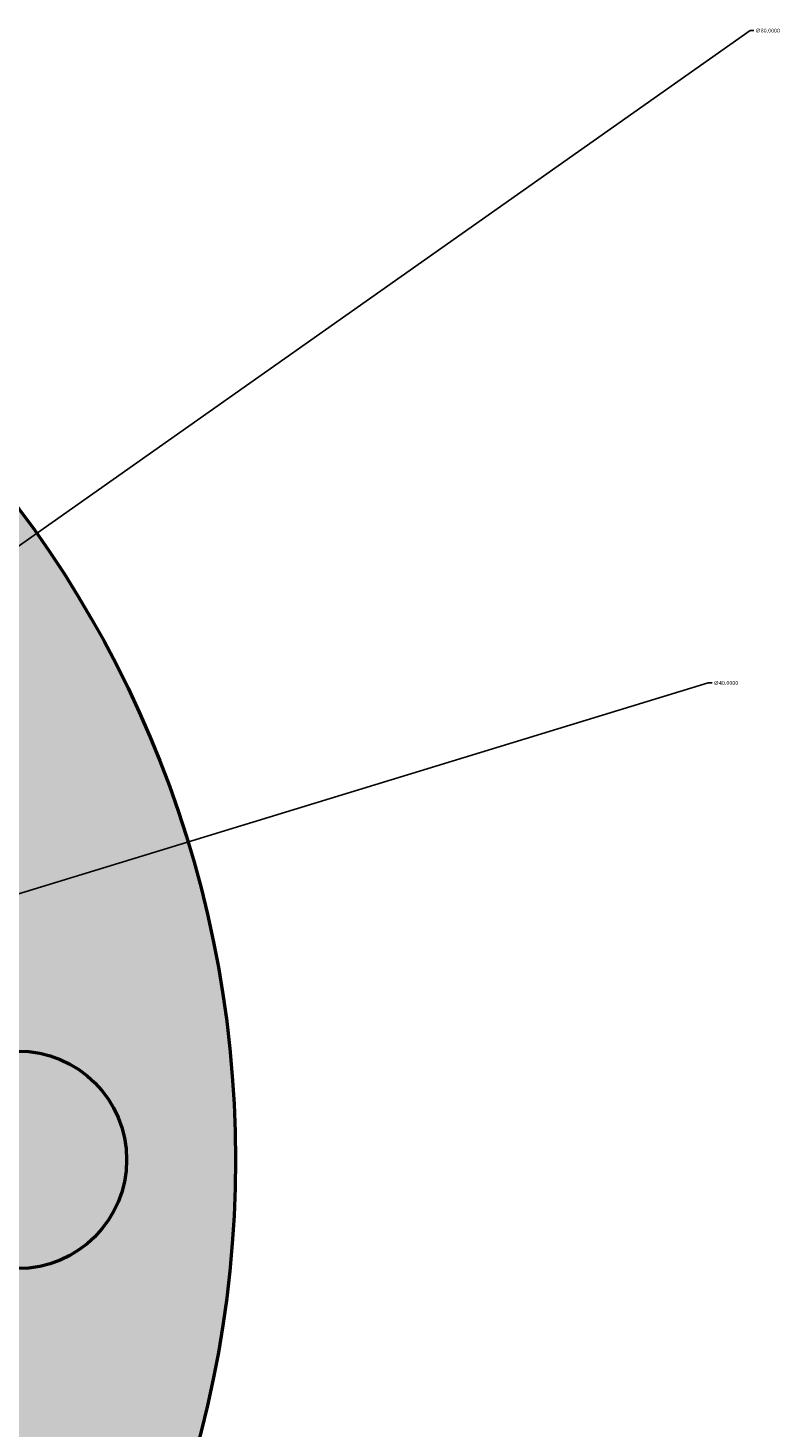
# Model space of a CAD drawing. Units: inches. Extents: x 139261 to 139415, y 52839 to 52963.
# Tile 20 of 20: x 139381 to 139415, y 52888 to 52952. Entities that reach past the tile are written whole.
import ezdxf

# ---------------------------------------------------------------- set-up
doc = ezdxf.new("R2010")
doc.units = ezdxf.units.IN
doc.header["$MEASUREMENT"] = 0
for name, color, linetype, lineweight in [('M-DIMS', 2, 'Continuous', 25), ('M-HATC', 8, 'Continuous', 18), ('M-OUTL', 7, 'Continuous', 50)]:
    doc.layers.add(name, color=color, linetype=linetype, lineweight=lineweight)
doc.styles.get("Standard").update_dxf_attribs({"font": 'arial.ttf'})
doc.dimstyles.get("Standard").update_dxf_attribs({"dimtxt": 0.18, "dimasz": 0.18, "dimexe": 0.18, "dimexo": 0.0625, "dimgap": 0.09, "dimtad": 0, "dimtih": 1, "dimtoh": 1, "dimdec": 4, "dimzin": 0, "dimdsep": 46, "dimtxsty": 'Standard', "dimcen": 0.09, "dimadec": 0, "dimazin": 0, "dimtfac": 1, "dimtdec": 4, "dimtofl": 0, "dimtmove": 0, "dimatfit": 3, "dimfxl": 1, "dimtolj": 1, "dimtzin": 0, "dimarcsym": 0})

# ---------------------------------------------------------------- blocks, each defined once
blk = doc.blocks.new('*U1')
blk.add_circle((0, 0), 5)
blk = doc.blocks.new('*U2')
at = {"layer": 'M-OUTL', "color": 0, "linetype": 'ByBlock', "lineweight": -2, "transparency": 16777216, "rotation": 270}
blk.add_blockref('*U1', (139380.357, 52900.217), dxfattribs=at)
blk = doc.blocks.new('*D3')
at = {"layer": 'Defpoints', "color": 0, "transparency": 16777216}
for p in [(139359.484, 52906.062), (139321.23, 52894.373)]:
    blk.add_point(p, dxfattribs=at)
at = {"layer": 'M-DIMS', "color": 0, "lineweight": -2, "transparency": 16777216}
for p, q in [((139412.091, 52922.136), (139359.656, 52906.115)), ((139412.271, 52922.136), (139412.091, 52922.136)), ((139340.267, 52900.217), (139340.447, 52900.217)), ((139340.357, 52900.127), (139340.357, 52900.307))]:
    blk.add_line(p, q, dxfattribs=at)
at = {"layer": 'M-DIMS', "color": 0, "transparency": 16777216}
blk.add_solid([(139359.647, 52906.143), (139359.665, 52906.086), (139359.484, 52906.062)], dxfattribs=at)
at = {"layer": 'M-DIMS', "color": 0, "transparency": 16777216, "insert": (139412.902, 52922.136), "char_height": 0.18, "attachment_point": 5}
blk.add_mtext('\\A1;∅40.0000', dxfattribs=at)
blk = doc.blocks.new('*D4')
at = {"layer": 'Defpoints', "color": 0, "transparency": 16777216}
for p in [(139373.053, 52923.26), (139307.661, 52877.175)]:
    blk.add_point(p, dxfattribs=at)
at = {"layer": 'M-DIMS', "color": 0, "lineweight": -2, "transparency": 16777216}
for p, q in [((139414.011, 52952.126), (139373.2, 52923.364)), ((139414.191, 52952.126), (139414.011, 52952.126)), ((139340.267, 52900.217), (139340.447, 52900.217)), ((139340.357, 52900.127), (139340.357, 52900.307))]:
    blk.add_line(p, q, dxfattribs=at)
blk.add_arc((139340.357, 52900.217), 40, 34.91676, 52.07712, dxfattribs=at)
at = {"layer": 'M-DIMS', "color": 0, "transparency": 16777216}
blk.add_solid([(139373.183, 52923.388), (139373.217, 52923.339), (139373.053, 52923.26)], dxfattribs=at)
at = {"layer": 'M-DIMS', "color": 0, "transparency": 16777216, "insert": (139414.822, 52952.126), "char_height": 0.18, "attachment_point": 5}
blk.add_mtext('\\A1;∅80.0000', dxfattribs=at)

msp = doc.modelspace()

# ---------------------------------------------------------------- hatches: boundary and pattern name
at = {"layer": 'M-HATC'}
h = msp.add_hatch(color=256, dxfattribs=at)
h.dxf.hatch_style = 1
h.paths.add_polyline_path([(139290.35689, 52900.21749, 1), (139390.35689, 52900.21749, 1)])
h.paths.add_polyline_path([(139335.36666, 52939.90499, -0.01563646), (139335.35689, 52940.21749, -1), (139345.35689, 52940.21749, -0.01563646), (139345.34711, 52939.90499, -0.13461315), (139364.89157, 52931.80941, -0.691035), (139373.64116, 52928.50176, -0.21521822), (139371.94881, 52924.75216, -0.13461315), (139380.04439, 52905.20771, -0.43265224), (139385.35689, 52900.21749, -0.43265224), (139380.04439, 52895.22726, -0.13461315), (139371.94881, 52875.68281, -0.21521822), (139373.64116, 52871.93321, -0.691035), (139364.89157, 52868.62556, -0.13461315), (139345.34711, 52860.52999, -0.01563646), (139345.35689, 52860.21749, -1), (139335.35689, 52860.21749, -0.01563646), (139335.36666, 52860.52999, -0.13461315), (139315.82221, 52868.62556, -0.691035), (139307.07262, 52871.93321, -0.21521822), (139308.76496, 52875.68281, -0.13461315), (139300.66939, 52895.22726, -0.43265224), (139295.35689, 52900.21749, -0.43265224), (139300.66939, 52905.20771, -0.13461315), (139308.76496, 52924.75216, -0.21521822), (139307.07262, 52928.50176, -0.691035), (139315.82221, 52931.80941, -0.13461315)], flags=16)
h.paths.add_polyline_path([(139365.35689, 52900.21749, -1), (139315.35689, 52900.21749, -1)], flags=0)
h.paths.add_polyline_path([(139323.71474, 52911.30978), (139356.99903, 52911.30978, -0.3027197), (139356.99903, 52889.12519), (139323.71474, 52889.12519, -0.3027197)], flags=0)
h.paths.add_polyline_path([(139364.89157, 52931.80941, 0.13461315), (139345.34711, 52939.90499, -0.93933644), (139335.36666, 52939.90499, 0.13461315), (139315.82221, 52931.80941, -0.18270763), (139317.07262, 52928.50176, -0.64579494), (139308.76496, 52924.75216, 0.13461315), (139300.66939, 52905.20771, -0.39601219), (139305.35689, 52900.21749, -0.39601219), (139300.66939, 52895.22726, 0.13461315), (139308.76496, 52875.68281, -0.64579494), (139317.07262, 52871.93321, -0.18270763), (139315.82221, 52868.62556, 0.13461315), (139335.36666, 52860.52999, -0.93933644), (139345.34711, 52860.52999, 0.13461315), (139364.89157, 52868.62556, -0.18270763), (139363.64116, 52871.93321, -0.64579494), (139371.94881, 52875.68281, 0.13461315), (139380.04439, 52895.22726, -0.39601219), (139375.35689, 52900.21749, -0.39601219), (139380.04439, 52905.20771, 0.13461315), (139371.94881, 52924.75216, -0.64579494), (139363.64116, 52928.50176, -0.18270763)], flags=0)
h = msp.add_hatch(color=256, dxfattribs=at)
h.dxf.hatch_style = 1
h.set_gradient(color1=(205, 105, 40), tint=1)
h.paths.add_polyline_path([(139335.35689, 52940.21749, 1), (139345.35689, 52940.21749, 1)])
h.paths.add_polyline_path([(139307.07262, 52928.50176, 1), (139317.07262, 52928.50176, 1)])
h.paths.add_polyline_path([(139295.35689, 52900.21749, 1), (139305.35689, 52900.21749, 1)])
h.paths.add_polyline_path([(139307.07262, 52871.93321, 1), (139317.07262, 52871.93321, 1)])
h.paths.add_polyline_path([(139345.35689, 52860.21749, 1), (139335.35689, 52860.21749, 1)])
h.paths.add_polyline_path([(139363.64116, 52871.93321, 1), (139373.64116, 52871.93321, 1)])
h.paths.add_polyline_path([(139375.35689, 52900.21749, 1), (139385.35689, 52900.21749, 1)])
h.paths.add_polyline_path([(139363.64116, 52928.50176, 1), (139373.64116, 52928.50176, 1)])

# ---------------------------------------------------------------- linework, layer by layer
at = {"layer": 'M-OUTL'}
msp.add_circle((139340.35689, 52900.21749), 50, dxfattribs=at)

# ---------------------------------------------------------------- block references
msp.add_blockref('*U2', (0, 0), dxfattribs=at)

# ---------------------------------------------------------------- dimensions: what is measured, and where the dimension line sits
at = {"layer": 'M-DIMS'}
for p1, p2, picture, middle in [((139307.66087, 52877.17469), (139373.0529, 52923.26028), '*D4', (139414.82217, 52952.12585)), ((139321.22987, 52894.37307), (139359.4839, 52906.0619), '*D3', (139412.90184, 52922.13633))]:
    dim = msp.add_diameter_dim_2p(p1=p1, p2=p2, dimstyle='Standard', override={"dimclrd": 0, "dimclre": 0, "dimclrt": 0}, dxfattribs=at)
    dim.commit()
    dim.dimension.update_dxf_attribs({"geometry": picture, "text_midpoint": middle, "dimtype": 163})

doc.saveas('drawing.dxf')
